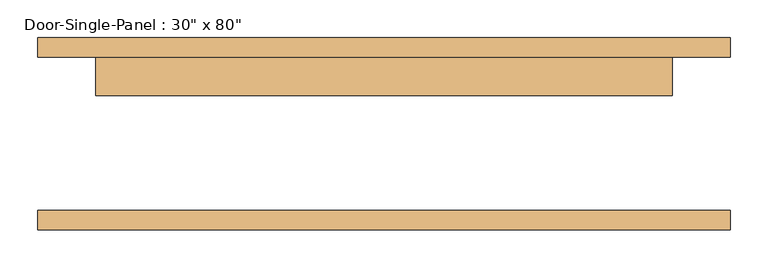
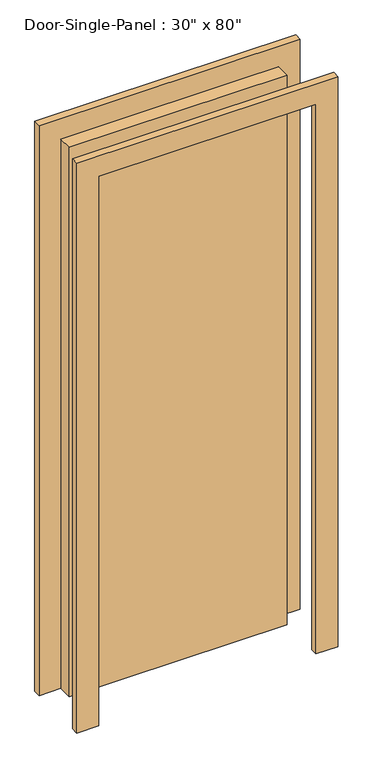
"""IFC4 building model written with IfcOpenShell, lengths in millimetres: door geometry."""

from ifc_helpers import new_model, si_unit, frame, origin, origin_with_axes, place, context, project, spatial, polyline, outline, extrude, source, transform, mapped, element, save


def door_1a782ffc(model_context):
    return source(origin(), model_context, "Body", "SweptSolid", [
        extrude(outline(polyline([(381.0, 50.8), (-381.0, 50.8), (-381.0, 101.6), (381.0, 101.6), (381.0, 50.8)])), origin_with_axes(), (0.0, 0.0, 1.0), 2032.0),
        extrude(outline(polyline([(2108.2, -457.2), (0.0, -457.2), (0.0, -381.0), (2032.0, -381.0), (2032.0, 381.0), (0.0, 381.0), (0.0, 457.2), (2108.2, 457.2), (2108.2, -457.2)])), frame((0.0, 101.6, 0.0), z_axis=(0.0, 1.0, 0.0), x_axis=(0.0, 0.0, 1.0)), (0.0, 0.0, 1.0), 25.4),
        extrude(outline(polyline([(2108.2, 457.2), (2108.2, -457.2), (0.0, -457.2), (0.0, -381.0), (2032.0, -381.0), (2032.0, 381.0), (0.0, 381.0), (0.0, 457.2), (2108.2, 457.2)])), frame((0.0, -127.0, 0.0), z_axis=(0.0, 1.0, 0.0), x_axis=(0.0, 0.0, 1.0)), (0.0, 0.0, 1.0), 25.4),
    ])


if __name__ == "__main__":
    model = new_model("IFC4")
    model_context = context("Model", 3, world=origin())
    ifc_project = project(units=[si_unit("LENGTHUNIT", "METRE", prefix="MILLI")], contexts=[model_context])
    site = spatial("IfcSite", under=ifc_project)
    building = spatial("IfcBuilding", under=site)
    placement = place(None, origin())
    door_shape = door_1a782ffc(model_context)
    element("IfcDoor", 1, ObjectType="Door-Single-Panel : 30\" x 80\"", at=placement, inside=building, context=model_context, shape_type="MappedRepresentation", body=[
        mapped(door_shape, transform((0.0, 0.0, 0.0), x_axis=(1.0, 0.0, 0.0), y_axis=(0.0, 1.0, 0.0), z_axis=(0.0, 0.0, 1.0))),
    ])
    save(model, "model.ifc")

# Revit data of these elements
# Type "Door-Single-Panel : 30\" x 80\""
#   Type Mark = "8"
#   Construction Type Id = "DOOR"
#   Assembly Code = "C1020300"
#   Analytic Construction = "Wooden"
#   Thickness = 0' - 2"
#   Thermal Resistance (R) = 2.5876 (h·ft²·°F)/BTU
#   Swing Angle [instance default] = 90.00°
#   Heat Transfer Coefficient (U) = 0.3865 BTU/(h·ft²·°F)
#   Height = 6' - 8"
#   Trim Projection Ext = 0' - 1"
#   Trim Projection Int = 0' - 1"
#   Trim Width = 0' - 3"
#   Width = 2' - 6"
#   Define Thermal Properties by = 1
#   Panel Material = Wood - Birch - Solid Stained Light Low Gloss
#   Trim Material = Paint - Sienna
#   Visual Light Transmittance = 0
#   Solar Heat Gain Coefficient = 0
#   Function = (empty or 0)
#   Wall Closure = (empty or 0)
# Element 1 (IfcDoor, "Door-Single-Panel : 30\" x 80\"")
#   Materials on its faces: "Paint - Sienna", "Wood - Birch - Solid Stained Light Low Gloss"
# Materials
#   "Wood - Birch - Solid Stained Light Low Gloss": class "Wood", colour RGB 210 159 95, transparency 0, Cost = 0
#   "Paint - Sienna": colour RGB 118 70 51, transparency 0, Cost = 0
